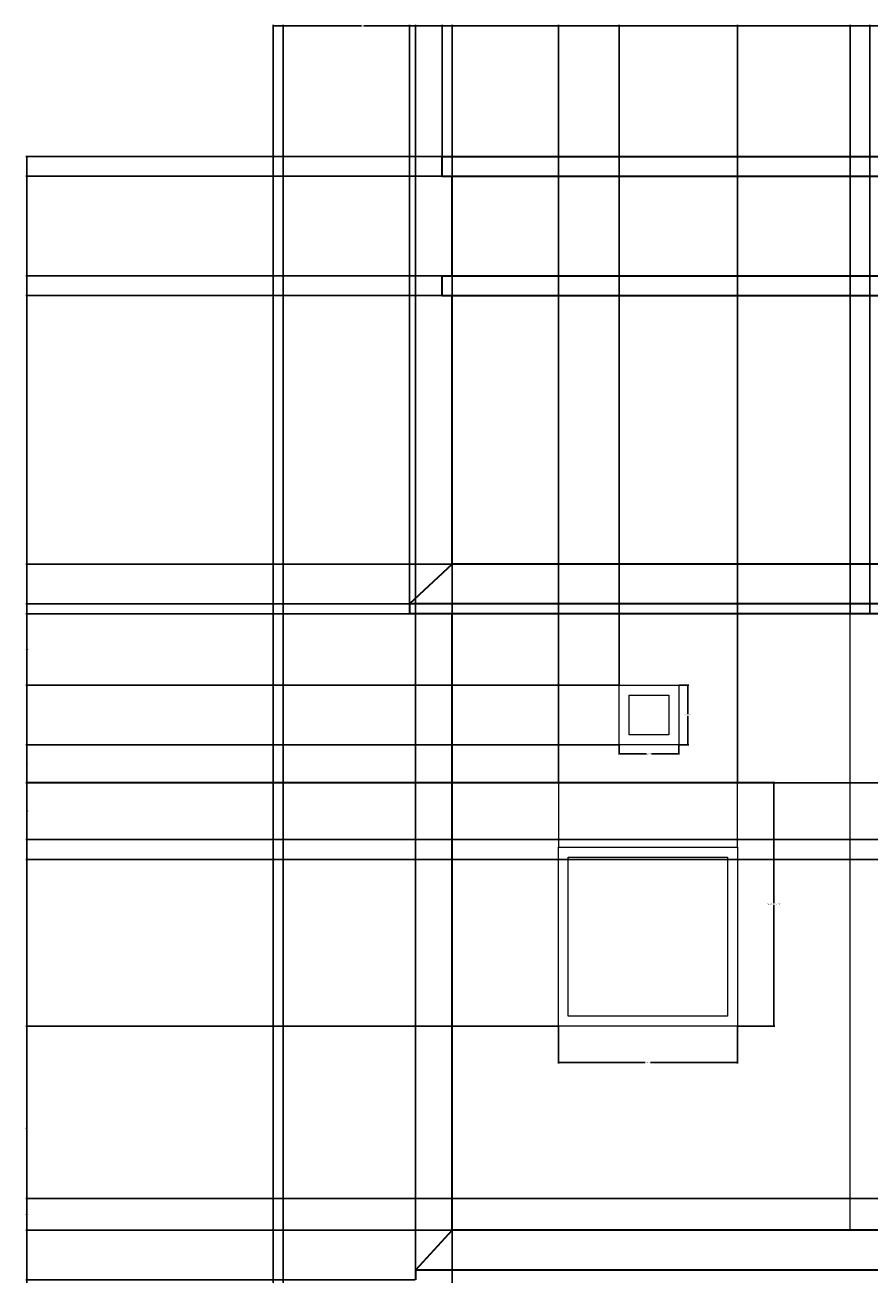
# Model space of a CAD drawing. Units: inches. Extents: x 1817 to 2378, y 1915 to 2370.
# Tile 4 of 8: x 1817 to 1987, y 2119 to 2370. Entities that reach past the tile are written whole.
import ezdxf

# ---------------------------------------------------------------- set-up
doc = ezdxf.new("R2010")
doc.units = ezdxf.units.IN
for name, color, linetype, lineweight in [('A-ANNO-DIMS', 2, 'Continuous', 18), ('A-ELEV', 7, 'Continuous', 35), ('A-GLAZ', 4, 'Continuous', 18), ('P-PIPE', 6, 'Continuous', 18)]:
    doc.layers.add(name, color=color, linetype=linetype, lineweight=lineweight)
doc.styles.get("Standard").update_dxf_attribs({"font": 'arial.ttf'})
doc.dimstyles.get("Standard").update_dxf_attribs({"dimtxt": 0.18, "dimasz": 0.18, "dimexe": 0.18, "dimexo": 0.0625, "dimgap": 0.09, "dimtad": 0, "dimtih": 1, "dimtoh": 1, "dimdec": 4, "dimzin": 0, "dimdsep": 46, "dimtxsty": 'Standard', "dimcen": 0.09, "dimadec": 0, "dimazin": 0, "dimtfac": 1, "dimtdec": 4, "dimtofl": 0, "dimtmove": 0, "dimatfit": 3, "dimfxl": 1, "dimtolj": 1, "dimtzin": 0, "dimarcsym": 0})

# ---------------------------------------------------------------- blocks, each defined once
blk = doc.blocks.new('WIN-SQ-900')
for points in [[(1924.43, 2204.58), (1960.43, 2204.58), (1960.43, 2217.58), (1924.43, 2217.58)], [(1924.43, 2204.58), (1960.43, 2204.58), (1960.43, 2168.58), (1924.43, 2168.58)], [(1926.43, 2202.58), (1958.43, 2202.58), (1958.43, 2170.58), (1926.43, 2170.58)]]:
    blk.add_lwpolyline(points, close=True)
blk = doc.blocks.new('VENT-300')
for points in [[(1936.66, 2237.16), (1948.66, 2237.16), (1948.66, 2225.16), (1936.66, 2225.16)], [(1938.66, 2235.16), (1946.66, 2235.16), (1946.66, 2227.16), (1938.66, 2227.16)]]:
    blk.add_lwpolyline(points, close=True)
blk = doc.blocks.new('*D4')
at = {"layer": 'A-ANNO-DIMS', "color": 0, "lineweight": -2, "transparency": 16777216}
for p, q in [((1960.49, 2217.58), (1967.96, 2217.58)), ((1967.78, 2217.4), (1967.78, 2193.27)), ((1967.78, 2168.76), (1967.78, 2192.89)), ((1960.49, 2168.58), (1967.96, 2168.58))]:
    blk.add_line(p, q, dxfattribs=at)
at = {"layer": 'A-ANNO-DIMS', "color": 0, "transparency": 16777216}
for points in [[(1967.75, 2217.4), (1967.81, 2217.4), (1967.78, 2217.58)], [(1967.75, 2168.76), (1967.81, 2168.76), (1967.78, 2168.58)]]:
    blk.add_solid(points, dxfattribs=at)
at = {"layer": 'Defpoints', "color": 0, "transparency": 16777216}
for p in [(1960.43, 2217.58), (1967.78, 2217.58), (1960.43, 2168.58)]:
    blk.add_point(p, dxfattribs=at)
at = {"layer": 'A-ANNO-DIMS', "color": 0, "transparency": 16777216, "insert": (1967.78, 2193.08), "char_height": 0.18, "attachment_point": 5}
blk.add_mtext('\\A1;SQUARE WINDOW 49 TYP.', dxfattribs=at)
blk = doc.blocks.new('*D5')
at = {"layer": 'A-ANNO-DIMS', "color": 0, "lineweight": -2, "transparency": 16777216}
for p, q in [((1924.43, 2168.52), (1924.43, 2161.05)), ((1960.43, 2168.52), (1960.43, 2161.05)), ((1924.61, 2161.23), (1941.9, 2161.23)), ((1960.25, 2161.23), (1942.95, 2161.23))]:
    blk.add_line(p, q, dxfattribs=at)
at = {"layer": 'A-ANNO-DIMS', "color": 0, "transparency": 16777216}
for points in [[(1924.61, 2161.26), (1924.61, 2161.2), (1924.43, 2161.23)], [(1960.25, 2161.26), (1960.25, 2161.2), (1960.43, 2161.23)]]:
    blk.add_solid(points, dxfattribs=at)
at = {"layer": 'Defpoints', "color": 0, "transparency": 16777216}
for p in [(1924.43, 2168.58), (1960.43, 2168.58), (1960.43, 2161.23)]:
    blk.add_point(p, dxfattribs=at)
at = {"layer": 'A-ANNO-DIMS', "color": 0, "transparency": 16777216, "insert": (1942.43, 2161.23), "char_height": 0.18, "attachment_point": 5}
blk.add_mtext('\\A1;36 TYP.', dxfattribs=at)
blk = doc.blocks.new('*D6')
at = {"layer": 'A-ANNO-DIMS', "color": 0, "lineweight": -2, "transparency": 16777216}
for p, q in [((1948.73, 2237.16), (1950.64, 2237.16)), ((1950.46, 2236.98), (1950.46, 2231.34)), ((1950.46, 2225.34), (1950.46, 2230.98)), ((1948.73, 2225.16), (1950.64, 2225.16))]:
    blk.add_line(p, q, dxfattribs=at)
at = {"layer": 'A-ANNO-DIMS', "color": 0, "transparency": 16777216}
for points in [[(1950.43, 2236.98), (1950.49, 2236.98), (1950.46, 2237.16)], [(1950.43, 2225.34), (1950.49, 2225.34), (1950.46, 2225.16)]]:
    blk.add_solid(points, dxfattribs=at)
at = {"layer": 'Defpoints', "color": 0, "transparency": 16777216}
for p in [(1948.66, 2237.16), (1950.46, 2237.16), (1948.66, 2225.16)]:
    blk.add_point(p, dxfattribs=at)
at = {"layer": 'A-ANNO-DIMS', "color": 0, "transparency": 16777216, "insert": (1950.46, 2231.16), "char_height": 0.18, "attachment_point": 5}
blk.add_mtext('\\A1;VENT 12 TYP.', dxfattribs=at)
blk = doc.blocks.new('*D7')
at = {"layer": 'A-ANNO-DIMS', "color": 0, "lineweight": -2, "transparency": 16777216}
for p, q in [((1936.66, 2225.1), (1936.66, 2223.18)), ((1936.84, 2223.36), (1942.15, 2223.36)), ((1948.48, 2223.36), (1943.18, 2223.36)), ((1948.66, 2225.1), (1948.66, 2223.18))]:
    blk.add_line(p, q, dxfattribs=at)
at = {"layer": 'A-ANNO-DIMS', "color": 0, "transparency": 16777216}
for points in [[(1936.84, 2223.39), (1936.84, 2223.33), (1936.66, 2223.36)], [(1948.48, 2223.39), (1948.48, 2223.33), (1948.66, 2223.36)]]:
    blk.add_solid(points, dxfattribs=at)
at = {"layer": 'Defpoints', "color": 0, "transparency": 16777216}
for p in [(1936.66, 2225.16), (1948.66, 2225.16), (1948.66, 2223.36)]:
    blk.add_point(p, dxfattribs=at)
at = {"layer": 'A-ANNO-DIMS', "color": 0, "transparency": 16777216, "insert": (1942.66, 2223.36), "char_height": 0.18, "attachment_point": 5}
blk.add_mtext('\\A1;12 TYP.', dxfattribs=at)
blk = doc.blocks.new('*D10')
at = {"layer": 'A-ANNO-DIMS', "color": 0, "lineweight": -2, "transparency": 16777216}
for p, q in [((1867.08, 2019.57), (1867.08, 2369.94)), ((1867.26, 2369.76), (1884.87, 2369.76)), ((1902.9, 2369.76), (1885.3, 2369.76)), ((1903.08, 2019.57), (1903.08, 2369.94))]:
    blk.add_line(p, q, dxfattribs=at)
at = {"layer": 'A-ANNO-DIMS', "color": 0, "transparency": 16777216}
for points in [[(1867.26, 2369.79), (1867.26, 2369.73), (1867.08, 2369.76)], [(1902.9, 2369.79), (1902.9, 2369.73), (1903.08, 2369.76)]]:
    blk.add_solid(points, dxfattribs=at)
at = {"layer": 'Defpoints', "color": 0, "transparency": 16777216}
for p in [(1903.08, 2369.76), (1867.08, 2019.51), (1903.08, 2019.51)]:
    blk.add_point(p, dxfattribs=at)
at = {"layer": 'A-ANNO-DIMS', "color": 0, "transparency": 16777216, "insert": (1885.08, 2369.76), "char_height": 0.18, "attachment_point": 5}
blk.add_mtext('\\A1;36', dxfattribs=at)
blk = doc.blocks.new('*D11')
at = {"layer": 'A-ANNO-DIMS', "color": 0, "lineweight": -2, "transparency": 16777216}
for p, q in [((1895.7, 2119.57), (1895.7, 2369.94)), ((1895.88, 2369.76), (1899, 2369.76)), ((1902.9, 2369.76), (1899.78, 2369.76)), ((1903.08, 2127.57), (1903.08, 2369.94))]:
    blk.add_line(p, q, dxfattribs=at)
at = {"layer": 'A-ANNO-DIMS', "color": 0, "transparency": 16777216}
for points in [[(1895.88, 2369.79), (1895.88, 2369.73), (1895.7, 2369.76)], [(1902.9, 2369.79), (1902.9, 2369.73), (1903.08, 2369.76)]]:
    blk.add_solid(points, dxfattribs=at)
at = {"layer": 'Defpoints', "color": 0, "transparency": 16777216}
for p in [(1903.08, 2369.76), (1903.08, 2127.51), (1895.7, 2119.51)]:
    blk.add_point(p, dxfattribs=at)
at = {"layer": 'A-ANNO-DIMS', "color": 0, "transparency": 16777216, "insert": (1899.39, 2369.76), "char_height": 0.18, "attachment_point": 5}
blk.add_mtext('\\A1;7.389', dxfattribs=at)
blk = doc.blocks.new('*D23')
at = {"layer": 'A-ANNO-DIMS', "color": 0, "lineweight": -2, "transparency": 16777216}
for p, q in [((2320.11, 2156.45), (2320.11, 1915.08)), ((1867.08, 1965.45), (1867.08, 1915.08)), ((1867.26, 1915.26), (2093.3, 1915.26)), ((2319.93, 1915.26), (2093.89, 1915.26))]:
    blk.add_line(p, q, dxfattribs=at)
at = {"layer": 'A-ANNO-DIMS', "color": 0, "transparency": 16777216}
for points in [[(1867.26, 1915.29), (1867.26, 1915.23), (1867.08, 1915.26)], [(2319.93, 1915.29), (2319.93, 1915.23), (2320.11, 1915.26)]]:
    blk.add_solid(points, dxfattribs=at)
at = {"layer": 'Defpoints', "color": 0, "transparency": 16777216}
for p in [(2320.11, 2156.51), (1867.08, 1965.51), (2320.11, 1915.26)]:
    blk.add_point(p, dxfattribs=at)
at = {"layer": 'A-ANNO-DIMS', "color": 0, "transparency": 16777216, "insert": (2093.6, 1915.26), "char_height": 0.18, "attachment_point": 5}
blk.add_mtext('\\A1;453', dxfattribs=at)
blk = doc.blocks.new('*D25')
at = {"layer": 'A-ANNO-DIMS', "color": 0, "lineweight": -2, "transparency": 16777216}
for p, q in [((1903.08, 2127.57), (1903.08, 2369.94)), ((1903.26, 2369.76), (1913.36, 2369.76)), ((1924.25, 2369.76), (1914.15, 2369.76)), ((1924.43, 2217.64), (1924.43, 2369.94))]:
    blk.add_line(p, q, dxfattribs=at)
at = {"layer": 'A-ANNO-DIMS', "color": 0, "transparency": 16777216}
for points in [[(1903.26, 2369.79), (1903.26, 2369.73), (1903.08, 2369.76)], [(1924.25, 2369.79), (1924.25, 2369.73), (1924.43, 2369.76)]]:
    blk.add_solid(points, dxfattribs=at)
at = {"layer": 'Defpoints', "color": 0, "transparency": 16777216}
for p in [(1924.43, 2369.76), (1924.43, 2217.58), (1903.08, 2127.51)]:
    blk.add_point(p, dxfattribs=at)
at = {"layer": 'A-ANNO-DIMS', "color": 0, "transparency": 16777216, "insert": (1913.76, 2369.76), "char_height": 0.18, "attachment_point": 5}
blk.add_mtext('\\A1;21.34', dxfattribs=at)
blk = doc.blocks.new('*D26')
at = {"layer": 'A-ANNO-DIMS', "color": 0, "lineweight": -2, "transparency": 16777216}
for p, q in [((1924.43, 2217.64), (1924.43, 2369.94)), ((1924.61, 2369.76), (1930.16, 2369.76)), ((1936.48, 2369.76), (1930.93, 2369.76)), ((1936.66, 2237.22), (1936.66, 2369.94))]:
    blk.add_line(p, q, dxfattribs=at)
at = {"layer": 'A-ANNO-DIMS', "color": 0, "transparency": 16777216}
for points in [[(1924.61, 2369.79), (1924.61, 2369.73), (1924.43, 2369.76)], [(1936.48, 2369.79), (1936.48, 2369.73), (1936.66, 2369.76)]]:
    blk.add_solid(points, dxfattribs=at)
at = {"layer": 'Defpoints', "color": 0, "transparency": 16777216}
for p in [(1936.66, 2369.76), (1936.66, 2237.16), (1924.43, 2217.58)]:
    blk.add_point(p, dxfattribs=at)
at = {"layer": 'A-ANNO-DIMS', "color": 0, "transparency": 16777216, "insert": (1930.55, 2369.76), "char_height": 0.18, "attachment_point": 5}
blk.add_mtext('\\A1;12.24', dxfattribs=at)
blk = doc.blocks.new('*D27')
at = {"layer": 'A-ANNO-DIMS', "color": 0, "lineweight": -2, "transparency": 16777216}
for p, q in [((1936.66, 2237.22), (1936.66, 2369.94)), ((1936.84, 2369.76), (1948.15, 2369.76)), ((1960.25, 2369.76), (1948.94, 2369.76)), ((1960.43, 2217.64), (1960.43, 2369.94))]:
    blk.add_line(p, q, dxfattribs=at)
at = {"layer": 'A-ANNO-DIMS', "color": 0, "transparency": 16777216}
for points in [[(1936.84, 2369.79), (1936.84, 2369.73), (1936.66, 2369.76)], [(1960.25, 2369.79), (1960.25, 2369.73), (1960.43, 2369.76)]]:
    blk.add_solid(points, dxfattribs=at)
at = {"layer": 'Defpoints', "color": 0, "transparency": 16777216}
for p in [(1960.43, 2369.76), (1936.66, 2237.16), (1960.43, 2217.58)]:
    blk.add_point(p, dxfattribs=at)
at = {"layer": 'A-ANNO-DIMS', "color": 0, "transparency": 16777216, "insert": (1948.55, 2369.76), "char_height": 0.18, "attachment_point": 5}
blk.add_mtext('\\A1;23.76', dxfattribs=at)
blk = doc.blocks.new('*D28')
at = {"layer": 'A-ANNO-DIMS', "color": 0, "lineweight": -2, "transparency": 16777216}
for p, q in [((1960.43, 2217.64), (1960.43, 2369.94)), ((1960.61, 2369.76), (1971.36, 2369.76)), ((1982.9, 2369.76), (1972.15, 2369.76)), ((1983.08, 2251.57), (1983.08, 2369.94))]:
    blk.add_line(p, q, dxfattribs=at)
at = {"layer": 'A-ANNO-DIMS', "color": 0, "transparency": 16777216}
for points in [[(1960.61, 2369.79), (1960.61, 2369.73), (1960.43, 2369.76)], [(1982.9, 2369.79), (1982.9, 2369.73), (1983.08, 2369.76)]]:
    blk.add_solid(points, dxfattribs=at)
at = {"layer": 'Defpoints', "color": 0, "transparency": 16777216}
for p in [(1983.08, 2369.76), (1983.08, 2251.51), (1960.43, 2217.58)]:
    blk.add_point(p, dxfattribs=at)
at = {"layer": 'A-ANNO-DIMS', "color": 0, "transparency": 16777216, "insert": (1971.76, 2369.76), "char_height": 0.18, "attachment_point": 5}
blk.add_mtext('\\A1;22.66', dxfattribs=at)
blk = doc.blocks.new('*D29')
at = {"layer": 'A-ANNO-DIMS', "color": 0, "lineweight": -2, "transparency": 16777216}
for p, q in [((1983.08, 2251.57), (1983.08, 2369.94)), ((1983.26, 2369.76), (1984.93, 2369.76)), ((1986.9, 2369.76), (1985.24, 2369.76)), ((1987.08, 2251.57), (1987.08, 2369.94))]:
    blk.add_line(p, q, dxfattribs=at)
at = {"layer": 'A-ANNO-DIMS', "color": 0, "transparency": 16777216}
for points in [[(1983.26, 2369.79), (1983.26, 2369.73), (1983.08, 2369.76)], [(1986.9, 2369.79), (1986.9, 2369.73), (1987.08, 2369.76)]]:
    blk.add_solid(points, dxfattribs=at)
at = {"layer": 'Defpoints', "color": 0, "transparency": 16777216}
for p in [(1987.08, 2369.76), (1983.08, 2251.51), (1987.08, 2251.51)]:
    blk.add_point(p, dxfattribs=at)
at = {"layer": 'A-ANNO-DIMS', "color": 0, "transparency": 16777216, "insert": (1985.08, 2369.76), "char_height": 0.18, "attachment_point": 5}
blk.add_mtext('\\A1;4', dxfattribs=at)
blk = doc.blocks.new('*D30')
at = {"layer": 'A-ANNO-DIMS', "color": 0, "lineweight": -2, "transparency": 16777216}
for p, q in [((1987.08, 2251.57), (1987.08, 2369.94)), ((1987.26, 2369.76), (1996.86, 2369.76)), ((2006.9, 2369.76), (1997.31, 2369.76)), ((2007.08, 2251.57), (2007.08, 2369.94))]:
    blk.add_line(p, q, dxfattribs=at)
at = {"layer": 'A-ANNO-DIMS', "color": 0, "transparency": 16777216}
for points in [[(1987.26, 2369.79), (1987.26, 2369.73), (1987.08, 2369.76)], [(2006.9, 2369.79), (2006.9, 2369.73), (2007.08, 2369.76)]]:
    blk.add_solid(points, dxfattribs=at)
at = {"layer": 'Defpoints', "color": 0, "transparency": 16777216}
for p in [(2007.08, 2369.76), (1987.08, 2251.51), (2007.08, 2251.51)]:
    blk.add_point(p, dxfattribs=at)
at = {"layer": 'A-ANNO-DIMS', "color": 0, "transparency": 16777216, "insert": (1997.08, 2369.76), "char_height": 0.18, "attachment_point": 5}
blk.add_mtext('\\A1;20', dxfattribs=at)
blk = doc.blocks.new('*D42')
at = {"layer": 'A-ANNO-DIMS', "color": 0, "lineweight": -2, "transparency": 16777216}
for p, q in [((1894.51, 2253.57), (1894.51, 2369.94)), ((1894.69, 2369.76), (1898.4, 2369.76)), ((1902.9, 2369.76), (1899.19, 2369.76)), ((1903.08, 2261.57), (1903.08, 2369.94))]:
    blk.add_line(p, q, dxfattribs=at)
at = {"layer": 'A-ANNO-DIMS', "color": 0, "transparency": 16777216}
for points in [[(1894.69, 2369.79), (1894.69, 2369.73), (1894.51, 2369.76)], [(1902.9, 2369.79), (1902.9, 2369.73), (1903.08, 2369.76)]]:
    blk.add_solid(points, dxfattribs=at)
at = {"layer": 'Defpoints', "color": 0, "transparency": 16777216}
for p in [(1903.08, 2369.76), (1903.08, 2261.51), (1894.51, 2253.51)]:
    blk.add_point(p, dxfattribs=at)
at = {"layer": 'A-ANNO-DIMS', "color": 0, "transparency": 16777216, "insert": (1898.8, 2369.76), "char_height": 0.18, "attachment_point": 5}
blk.add_mtext('\\A1;8.579', dxfattribs=at)
blk = doc.blocks.new('*D43')
at = {"layer": 'A-ANNO-DIMS', "color": 0, "lineweight": -2, "transparency": 16777216}
for p, q in [((1901.08, 2343.57), (1901.08, 2369.94)), ((1901.26, 2369.76), (1901.94, 2369.76)), ((1902.9, 2369.76), (1902.23, 2369.76)), ((1903.08, 2339.57), (1903.08, 2369.94))]:
    blk.add_line(p, q, dxfattribs=at)
at = {"layer": 'A-ANNO-DIMS', "color": 0, "transparency": 16777216}
for points in [[(1901.26, 2369.79), (1901.26, 2369.73), (1901.08, 2369.76)], [(1902.9, 2369.79), (1902.9, 2369.73), (1903.08, 2369.76)]]:
    blk.add_solid(points, dxfattribs=at)
at = {"layer": 'Defpoints', "color": 0, "transparency": 16777216}
for p in [(1903.08, 2369.76), (1901.08, 2343.51), (1903.08, 2339.51)]:
    blk.add_point(p, dxfattribs=at)
at = {"layer": 'A-ANNO-DIMS', "color": 0, "transparency": 16777216, "insert": (1902.08, 2369.76), "char_height": 0.18, "attachment_point": 5}
blk.add_mtext('\\A1;2', dxfattribs=at)
blk = doc.blocks.new('*D44')
at = {"layer": 'A-ANNO-DIMS', "color": 0, "lineweight": -2, "transparency": 16777216}
for p, q in [((1903.08, 2261.57), (1903.08, 2369.94)), ((1903.26, 2369.76), (1954.8, 2369.76)), ((2006.9, 2369.76), (1955.36, 2369.76)), ((2007.08, 2291.57), (2007.08, 2369.94))]:
    blk.add_line(p, q, dxfattribs=at)
at = {"layer": 'A-ANNO-DIMS', "color": 0, "transparency": 16777216}
for points in [[(1903.26, 2369.79), (1903.26, 2369.73), (1903.08, 2369.76)], [(2006.9, 2369.79), (2006.9, 2369.73), (2007.08, 2369.76)]]:
    blk.add_solid(points, dxfattribs=at)
at = {"layer": 'Defpoints', "color": 0, "transparency": 16777216}
for p in [(2007.08, 2369.76), (2007.08, 2291.51), (1903.08, 2261.51)]:
    blk.add_point(p, dxfattribs=at)
at = {"layer": 'A-ANNO-DIMS', "color": 0, "transparency": 16777216, "insert": (1955.08, 2369.76), "char_height": 0.18, "attachment_point": 5}
blk.add_mtext('\\A1;104', dxfattribs=at)
blk = doc.blocks.new('*D51')
at = {"layer": 'A-ANNO-DIMS', "color": 0, "lineweight": -2, "transparency": 16777216}
for p, q in [((2281.02, 2261.51), (1817.4, 2261.51)), ((1817.58, 2261.33), (1817.58, 2257.69)), ((1817.58, 2253.69), (1817.58, 2257.33)), ((2289.54, 2253.51), (1817.4, 2253.51))]:
    blk.add_line(p, q, dxfattribs=at)
at = {"layer": 'A-ANNO-DIMS', "color": 0, "transparency": 16777216}
for points in [[(1817.55, 2261.33), (1817.61, 2261.33), (1817.58, 2261.51)], [(1817.55, 2253.69), (1817.61, 2253.69), (1817.58, 2253.51)]]:
    blk.add_solid(points, dxfattribs=at)
at = {"layer": 'Defpoints', "color": 0, "transparency": 16777216}
for p in [(1817.58, 2261.51), (2281.08, 2261.51), (2289.61, 2253.51)]:
    blk.add_point(p, dxfattribs=at)
at = {"layer": 'A-ANNO-DIMS', "color": 0, "transparency": 16777216, "insert": (1817.58, 2257.51), "char_height": 0.18, "attachment_point": 5}
blk.add_mtext('\\A1;8', dxfattribs=at)
blk = doc.blocks.new('*D54')
at = {"layer": 'A-ANNO-DIMS', "color": 0, "lineweight": -2, "transparency": 16777216}
for p, q in [((1901.02, 2343.51), (1817.4, 2343.51)), ((1817.58, 2343.33), (1817.58, 2154.69)), ((1817.58, 1965.69), (1817.58, 2154.33)), ((1867.02, 1965.51), (1817.4, 1965.51))]:
    blk.add_line(p, q, dxfattribs=at)
at = {"layer": 'A-ANNO-DIMS', "color": 0, "transparency": 16777216}
for points in [[(1817.55, 2343.33), (1817.61, 2343.33), (1817.58, 2343.51)], [(1817.55, 1965.69), (1817.61, 1965.69), (1817.58, 1965.51)]]:
    blk.add_solid(points, dxfattribs=at)
at = {"layer": 'Defpoints', "color": 0, "transparency": 16777216}
for p in [(1817.58, 2343.51), (1901.08, 2343.51), (1867.08, 1965.51)]:
    blk.add_point(p, dxfattribs=at)
at = {"layer": 'A-ANNO-DIMS', "color": 0, "transparency": 16777216, "insert": (1817.58, 2154.51), "char_height": 0.18, "attachment_point": 5}
blk.add_mtext('\\A1;378', dxfattribs=at)
blk = doc.blocks.new('*D60')
at = {"layer": 'A-ANNO-DIMS', "color": 0, "lineweight": -2, "transparency": 16777216}
for p, q in [((1903.02, 2127.51), (1817.4, 2127.51)), ((1817.58, 2127.33), (1817.58, 2122.69)), ((1817.58, 2117.69), (1817.58, 2122.33)), ((1895.63, 2117.51), (1817.4, 2117.51))]:
    blk.add_line(p, q, dxfattribs=at)
at = {"layer": 'A-ANNO-DIMS', "color": 0, "transparency": 16777216}
for points in [[(1817.55, 2127.33), (1817.61, 2127.33), (1817.58, 2127.51)], [(1817.55, 2117.69), (1817.61, 2117.69), (1817.58, 2117.51)]]:
    blk.add_solid(points, dxfattribs=at)
at = {"layer": 'Defpoints', "color": 0, "transparency": 16777216}
for p in [(1817.58, 2127.51), (1903.08, 2127.51), (1895.7, 2117.51)]:
    blk.add_point(p, dxfattribs=at)
at = {"layer": 'A-ANNO-DIMS', "color": 0, "transparency": 16777216, "insert": (1817.58, 2122.51), "char_height": 0.18, "attachment_point": 5}
blk.add_mtext('\\A1;10', dxfattribs=at)
blk = doc.blocks.new('*D61')
at = {"layer": 'A-ANNO-DIMS', "color": 0, "lineweight": -2, "transparency": 16777216}
for p, q in [((1924.36, 2168.58), (1817.4, 2168.58)), ((1817.58, 2168.4), (1817.58, 2148.23)), ((1817.58, 2127.69), (1817.58, 2147.86)), ((1903.02, 2127.51), (1817.4, 2127.51))]:
    blk.add_line(p, q, dxfattribs=at)
at = {"layer": 'A-ANNO-DIMS', "color": 0, "transparency": 16777216}
for points in [[(1817.55, 2168.4), (1817.61, 2168.4), (1817.58, 2168.58)], [(1817.55, 2127.69), (1817.61, 2127.69), (1817.58, 2127.51)]]:
    blk.add_solid(points, dxfattribs=at)
at = {"layer": 'Defpoints', "color": 0, "transparency": 16777216}
for p in [(1817.58, 2168.58), (1924.43, 2168.58), (1903.08, 2127.51)]:
    blk.add_point(p, dxfattribs=at)
at = {"layer": 'A-ANNO-DIMS', "color": 0, "transparency": 16777216, "insert": (1817.58, 2148.05), "char_height": 0.18, "attachment_point": 5}
blk.add_mtext('\\A1;41.07', dxfattribs=at)
blk = doc.blocks.new('*D62')
at = {"layer": 'A-ANNO-DIMS', "color": 0, "lineweight": -2, "transparency": 16777216}
for p, q in [((1936.6, 2225.16), (1817.4, 2225.16)), ((1817.58, 2224.98), (1817.58, 2221.55)), ((1817.58, 2217.76), (1817.58, 2221.19)), ((1924.36, 2217.58), (1817.4, 2217.58))]:
    blk.add_line(p, q, dxfattribs=at)
at = {"layer": 'A-ANNO-DIMS', "color": 0, "transparency": 16777216}
for points in [[(1817.55, 2224.98), (1817.61, 2224.98), (1817.58, 2225.16)], [(1817.55, 2217.76), (1817.61, 2217.76), (1817.58, 2217.58)]]:
    blk.add_solid(points, dxfattribs=at)
at = {"layer": 'Defpoints', "color": 0, "transparency": 16777216}
for p in [(1817.58, 2225.16), (1936.66, 2225.16), (1924.43, 2217.58)]:
    blk.add_point(p, dxfattribs=at)
at = {"layer": 'A-ANNO-DIMS', "color": 0, "transparency": 16777216, "insert": (1817.58, 2221.37), "char_height": 0.18, "attachment_point": 5}
blk.add_mtext('\\A1;7.578', dxfattribs=at)
blk = doc.blocks.new('*D63')
at = {"layer": 'A-ANNO-DIMS', "color": 0, "lineweight": -2, "transparency": 16777216}
for p, q in [((1903.02, 2251.51), (1817.4, 2251.51)), ((1817.58, 2251.33), (1817.58, 2244.52)), ((1817.58, 2237.34), (1817.58, 2244.15)), ((1936.6, 2237.16), (1817.4, 2237.16))]:
    blk.add_line(p, q, dxfattribs=at)
at = {"layer": 'A-ANNO-DIMS', "color": 0, "transparency": 16777216}
for points in [[(1817.55, 2251.33), (1817.61, 2251.33), (1817.58, 2251.51)], [(1817.55, 2237.34), (1817.61, 2237.34), (1817.58, 2237.16)]]:
    blk.add_solid(points, dxfattribs=at)
at = {"layer": 'Defpoints', "color": 0, "transparency": 16777216}
for p in [(1817.58, 2251.51), (1903.08, 2251.51), (1936.66, 2237.16)]:
    blk.add_point(p, dxfattribs=at)
at = {"layer": 'A-ANNO-DIMS', "color": 0, "transparency": 16777216, "insert": (1817.58, 2244.33), "char_height": 0.18, "attachment_point": 5}
blk.add_mtext('\\A1;14.35', dxfattribs=at)
blk = doc.blocks.new('*D64')
at = {"layer": 'A-ANNO-DIMS', "color": 0, "lineweight": -2, "transparency": 16777216}
for p, q in [((1903.02, 2261.51), (1817.4, 2261.51)), ((1817.58, 2261.33), (1817.58, 2256.69)), ((1817.58, 2251.69), (1817.58, 2256.33)), ((1894.44, 2251.51), (1817.4, 2251.51))]:
    blk.add_line(p, q, dxfattribs=at)
at = {"layer": 'A-ANNO-DIMS', "color": 0, "transparency": 16777216}
for points in [[(1817.55, 2261.33), (1817.61, 2261.33), (1817.58, 2261.51)], [(1817.55, 2251.69), (1817.61, 2251.69), (1817.58, 2251.51)]]:
    blk.add_solid(points, dxfattribs=at)
at = {"layer": 'Defpoints', "color": 0, "transparency": 16777216}
for p in [(1817.58, 2261.51), (1903.08, 2261.51), (1894.51, 2251.51)]:
    blk.add_point(p, dxfattribs=at)
at = {"layer": 'A-ANNO-DIMS', "color": 0, "transparency": 16777216, "insert": (1817.58, 2256.51), "char_height": 0.18, "attachment_point": 5}
blk.add_mtext('\\A1;10', dxfattribs=at)
blk = doc.blocks.new('*D65')
at = {"layer": 'A-ANNO-DIMS', "color": 0, "lineweight": -2, "transparency": 16777216}
for p, q in [((1901.02, 2315.51), (1817.4, 2315.51)), ((1817.58, 2315.33), (1817.58, 2288.69)), ((1817.58, 2261.69), (1817.58, 2288.33)), ((1903.02, 2261.51), (1817.4, 2261.51))]:
    blk.add_line(p, q, dxfattribs=at)
at = {"layer": 'A-ANNO-DIMS', "color": 0, "transparency": 16777216}
for points in [[(1817.55, 2315.33), (1817.61, 2315.33), (1817.58, 2315.51)], [(1817.55, 2261.69), (1817.61, 2261.69), (1817.58, 2261.51)]]:
    blk.add_solid(points, dxfattribs=at)
at = {"layer": 'Defpoints', "color": 0, "transparency": 16777216}
for p in [(1817.58, 2315.51), (1901.08, 2315.51), (1903.08, 2261.51)]:
    blk.add_point(p, dxfattribs=at)
at = {"layer": 'A-ANNO-DIMS', "color": 0, "transparency": 16777216, "insert": (1817.58, 2288.51), "char_height": 0.18, "attachment_point": 5}
blk.add_mtext('\\A1;54', dxfattribs=at)
blk = doc.blocks.new('*D66')
at = {"layer": 'A-ANNO-DIMS', "color": 0, "lineweight": -2, "transparency": 16777216}
for p, q in [((1901.022352, 2319.508728), (1817.404024, 2319.508728)), ((1817.584024, 2319.328728), (1817.584024, 2317.688728)), ((1817.584024, 2315.688728), (1817.584024, 2317.328728)), ((1901.022352, 2315.508728), (1817.404024, 2315.508728))]:
    blk.add_line(p, q, dxfattribs=at)
at = {"layer": 'A-ANNO-DIMS', "color": 0, "transparency": 16777216}
for points in [[(1817.554024, 2319.328728), (1817.614024, 2319.328728), (1817.584024, 2319.508728)], [(1817.554024, 2315.688728), (1817.614024, 2315.688728), (1817.584024, 2315.508728)]]:
    blk.add_solid(points, dxfattribs=at)
at = {"layer": 'Defpoints', "color": 0, "transparency": 16777216}
for p in [(1817.584024, 2319.508728), (1901.084852, 2319.508728), (1901.084852, 2315.508728)]:
    blk.add_point(p, dxfattribs=at)
at = {"layer": 'A-ANNO-DIMS', "color": 0, "transparency": 16777216, "insert": (1817.584024, 2317.508728), "char_height": 0.18, "attachment_point": 5}
blk.add_mtext('\\A1;4', dxfattribs=at)
blk = doc.blocks.new('*D67')
at = {"layer": 'A-ANNO-DIMS', "color": 0, "lineweight": -2, "transparency": 16777216}
for p, q in [((1901.02, 2339.51), (1817.4, 2339.51)), ((1817.58, 2339.33), (1817.58, 2329.69)), ((1817.58, 2319.69), (1817.58, 2329.33)), ((1901.02, 2319.51), (1817.4, 2319.51))]:
    blk.add_line(p, q, dxfattribs=at)
at = {"layer": 'A-ANNO-DIMS', "color": 0, "transparency": 16777216}
for points in [[(1817.55, 2339.33), (1817.61, 2339.33), (1817.58, 2339.51)], [(1817.55, 2319.69), (1817.61, 2319.69), (1817.58, 2319.51)]]:
    blk.add_solid(points, dxfattribs=at)
at = {"layer": 'Defpoints', "color": 0, "transparency": 16777216}
for p in [(1817.58, 2339.51), (1901.08, 2339.51), (1901.08, 2319.51)]:
    blk.add_point(p, dxfattribs=at)
at = {"layer": 'A-ANNO-DIMS', "color": 0, "transparency": 16777216, "insert": (1817.58, 2329.51), "char_height": 0.18, "attachment_point": 5}
blk.add_mtext('\\A1;20', dxfattribs=at)
blk = doc.blocks.new('*D68')
at = {"layer": 'A-ANNO-DIMS', "color": 0, "lineweight": -2, "transparency": 16777216}
for p, q in [((1901.022352, 2343.508728), (1817.404024, 2343.508728)), ((1817.584024, 2343.328728), (1817.584024, 2341.688728)), ((1817.584024, 2339.688728), (1817.584024, 2341.328728)), ((1901.022352, 2339.508728), (1817.404024, 2339.508728))]:
    blk.add_line(p, q, dxfattribs=at)
at = {"layer": 'A-ANNO-DIMS', "color": 0, "transparency": 16777216}
for points in [[(1817.554024, 2343.328728), (1817.614024, 2343.328728), (1817.584024, 2343.508728)], [(1817.554024, 2339.688728), (1817.614024, 2339.688728), (1817.584024, 2339.508728)]]:
    blk.add_solid(points, dxfattribs=at)
at = {"layer": 'Defpoints', "color": 0, "transparency": 16777216}
for p in [(1817.584024, 2343.508728), (1901.084852, 2343.508728), (1901.084852, 2339.508728)]:
    blk.add_point(p, dxfattribs=at)
at = {"layer": 'A-ANNO-DIMS', "color": 0, "transparency": 16777216, "insert": (1817.584024, 2341.508728), "char_height": 0.18, "attachment_point": 5}
blk.add_mtext('\\A1;4', dxfattribs=at)
blk = doc.blocks.new('*D82')
at = {"layer": 'A-ANNO-DIMS', "color": 0, "lineweight": -2, "transparency": 16777216}
for p, q in [((2123.56, 2133.9), (1817.4, 2133.9)), ((1817.58, 2133.72), (1817.58, 2130.88)), ((1817.58, 2127.69), (1817.58, 2130.52)), ((2198.53, 2127.51), (1817.4, 2127.51))]:
    blk.add_line(p, q, dxfattribs=at)
at = {"layer": 'A-ANNO-DIMS', "color": 0, "transparency": 16777216}
for points in [[(1817.55, 2133.72), (1817.61, 2133.72), (1817.58, 2133.9)], [(1817.55, 2127.69), (1817.61, 2127.69), (1817.58, 2127.51)]]:
    blk.add_solid(points, dxfattribs=at)
at = {"layer": 'Defpoints', "color": 0, "transparency": 16777216}
for p in [(1817.58, 2133.9), (2123.62, 2133.9), (2198.59, 2127.51)]:
    blk.add_point(p, dxfattribs=at)
at = {"layer": 'A-ANNO-DIMS', "color": 0, "transparency": 16777216, "insert": (1817.58, 2130.7), "char_height": 0.18, "attachment_point": 5}
blk.add_mtext('\\A1;6.387', dxfattribs=at)
blk = doc.blocks.new('*D104')
at = {"layer": 'A-ANNO-DIMS', "color": 0, "lineweight": -2, "transparency": 16777216}
for p, q in [((2210.55, 2217.51), (1817.4, 2217.51)), ((1817.58, 2217.33), (1817.58, 2211.97)), ((1817.58, 2206.26), (1817.58, 2211.61)), ((2210.55, 2206.08), (1817.4, 2206.08))]:
    blk.add_line(p, q, dxfattribs=at)
at = {"layer": 'A-ANNO-DIMS', "color": 0, "transparency": 16777216}
for points in [[(1817.55, 2217.33), (1817.61, 2217.33), (1817.58, 2217.51)], [(1817.55, 2206.26), (1817.61, 2206.26), (1817.58, 2206.08)]]:
    blk.add_solid(points, dxfattribs=at)
at = {"layer": 'Defpoints', "color": 0, "transparency": 16777216}
for p in [(2210.62, 2217.51), (1817.58, 2206.08), (2210.62, 2206.08)]:
    blk.add_point(p, dxfattribs=at)
at = {"layer": 'A-ANNO-DIMS', "color": 0, "transparency": 16777216, "insert": (1817.58, 2211.79), "char_height": 0.18, "attachment_point": 5}
blk.add_mtext('\\A1;11.433', dxfattribs=at)
blk = doc.blocks.new('*D105')
at = {"layer": 'A-ANNO-DIMS', "color": 0, "lineweight": -2, "transparency": 16777216}
for p, q in [((2210.55, 2206.08), (1817.4, 2206.08)), ((1817.58, 2205.9), (1817.58, 2204.26)), ((1817.58, 2202.26), (1817.58, 2203.89)), ((2214.55, 2202.08), (1817.4, 2202.08))]:
    blk.add_line(p, q, dxfattribs=at)
at = {"layer": 'A-ANNO-DIMS', "color": 0, "transparency": 16777216}
for points in [[(1817.55, 2205.9), (1817.61, 2205.9), (1817.58, 2206.08)], [(1817.55, 2202.26), (1817.61, 2202.26), (1817.58, 2202.08)]]:
    blk.add_solid(points, dxfattribs=at)
at = {"layer": 'Defpoints', "color": 0, "transparency": 16777216}
for p in [(2210.62, 2206.08), (1817.58, 2202.08), (2214.62, 2202.08)]:
    blk.add_point(p, dxfattribs=at)
at = {"layer": 'A-ANNO-DIMS', "color": 0, "transparency": 16777216, "insert": (1817.58, 2204.08), "char_height": 0.18, "attachment_point": 5}
blk.add_mtext('\\A1;4.00', dxfattribs=at)
blk = doc.blocks.new('*D116')
at = {"layer": 'A-ANNO-DIMS', "color": 0, "lineweight": -2, "transparency": 16777216}
for p, q in [((1867.08, 2017.57), (1867.08, 2369.94)), ((1867.26, 2369.76), (1867.76, 2369.76)), ((1868.9, 2369.76), (1868.41, 2369.76)), ((1869.08, 2017.57), (1869.08, 2369.94))]:
    blk.add_line(p, q, dxfattribs=at)
at = {"layer": 'A-ANNO-DIMS', "color": 0, "transparency": 16777216}
for points in [[(1867.26, 2369.79), (1867.26, 2369.73), (1867.08, 2369.76)], [(1868.9, 2369.79), (1868.9, 2369.73), (1869.08, 2369.76)]]:
    blk.add_solid(points, dxfattribs=at)
at = {"layer": 'Defpoints', "color": 0, "transparency": 16777216}
for p in [(1869.08, 2369.76), (1867.08, 2017.51), (1869.08, 2017.51)]:
    blk.add_point(p, dxfattribs=at)
at = {"layer": 'A-ANNO-DIMS', "color": 0, "transparency": 16777216, "insert": (1868.08, 2369.76), "char_height": 0.18, "attachment_point": 5}
blk.add_mtext('\\A1;2.00', dxfattribs=at)
blk = doc.blocks.new('*D119')
at = {"layer": 'A-ANNO-DIMS', "color": 0, "lineweight": -2, "transparency": 16777216}
for p, q in [((1903.08, 1989.57), (1903.08, 2369.94)), ((1903.26, 2369.76), (2091.62, 2369.76)), ((2280.9, 2369.76), (2092.55, 2369.76)), ((2281.08, 1989.57), (2281.08, 2369.94))]:
    blk.add_line(p, q, dxfattribs=at)
at = {"layer": 'A-ANNO-DIMS', "color": 0, "transparency": 16777216}
for points in [[(1903.26, 2369.79), (1903.26, 2369.73), (1903.08, 2369.76)], [(2280.9, 2369.79), (2280.9, 2369.73), (2281.08, 2369.76)]]:
    blk.add_solid(points, dxfattribs=at)
at = {"layer": 'Defpoints', "color": 0, "transparency": 16777216}
for p in [(2281.08, 2369.76), (1903.08, 1989.51), (2281.08, 1989.51)]:
    blk.add_point(p, dxfattribs=at)
at = {"layer": 'A-ANNO-DIMS', "color": 0, "transparency": 16777216, "insert": (2092.08, 2369.76), "char_height": 0.18, "attachment_point": 5}
blk.add_mtext('\\A1;378.00', dxfattribs=at)

msp = doc.modelspace()

# ---------------------------------------------------------------- linework, layer by layer
at = {"layer": 'A-ELEV'}
for p, q in [((1901.0849, 2343.5087), (2127.0849, 2343.5087)), ((1901.0849, 2339.5087), (1901.0849, 2343.5087)), ((1901.0849, 2339.5087), (2127.0849, 2339.5087)), ((1903.0849, 2319.5087), (1903.0849, 2339.5087)), ((1901.0849, 2319.5087), (2009.0849, 2319.5087)), ((1901.0849, 2315.5087), (1901.0849, 2319.5087)), ((1901.0849, 2315.5087), (2009.0849, 2315.5087)), ((1903.0849, 2261.5087), (1903.0849, 2315.5087)), ((1903.0849, 2261.5087), (1894.506, 2253.5087)), ((2281.0849, 2261.5087), (1903.0849, 2261.5087)), ((2289.6055, 2253.5087), (1894.506, 2253.5087)), ((1894.506, 2253.5087), (1894.506, 2251.5087)), ((2289.6055, 2251.5087), (1894.506, 2251.5087)), ((1903.0849, 2127.5087), (1903.0849, 2251.5087)), ((1903.0849, 2127.5087), (1895.6961, 2119.5087)), ((2198.5896, 2127.5087), (1903.0849, 2127.5087)), ((2198.5896, 2119.5087), (1895.6961, 2119.5087)), ((1895.6961, 2119.5087), (1895.6961, 2117.5087))]:
    msp.add_line(p, q, dxfattribs=at)
at = {"layer": 'P-PIPE'}
msp.add_line((1983.0849, 2127.5087), (1983.0849, 2251.5087), dxfattribs=at)

# ---------------------------------------------------------------- block references
at = {"layer": 'A-GLAZ'}
for name in ['VENT-300', 'WIN-SQ-900']:
    msp.add_blockref(name, (0, 0), dxfattribs=at)

# ---------------------------------------------------------------- dimensions: what is measured, and where the dimension line sits
at = {"layer": 'A-ANNO-DIMS'}
for base, p1, p2, override, picture, middle in [((1903.0849, 2369.7587), (1867.0849, 2019.5087), (1903.0849, 2019.5087), {"dimdec": 0, "dimlfac": 1, "dimrnd": 0, "dimzin": 0, "dimdsep": 46, "dimlunit": 2}, '*D10', (1885.0849, 2369.7587)), ((1869.0849, 2369.7587), (1867.0849, 2017.5087), (1869.0849, 2017.5087), {"dimdec": 2, "dimlfac": 1, "dimrnd": 0, "dimzin": 0, "dimdsep": 46, "dimlunit": 2}, '*D116', (1868.0849, 2369.7587)), ((1903.0849, 2369.7587), (1894.506, 2253.5087), (1903.0849, 2261.5087), {"dimdec": 3, "dimlfac": 1, "dimrnd": 0, "dimzin": 0, "dimdsep": 46, "dimlunit": 2}, '*D42', (1898.7954, 2369.7587)), ((1903.0849, 2369.7587), (1895.6961, 2119.5087), (1903.0849, 2127.5087), {"dimdec": 3, "dimlfac": 1, "dimrnd": 0, "dimzin": 0, "dimdsep": 46, "dimlunit": 2}, '*D11', (1899.3905, 2369.7587)), ((1903.0849, 2369.7587), (1901.0849, 2343.5087), (1903.0849, 2339.5087), {"dimdec": 0, "dimlfac": 1, "dimrnd": 0, "dimzin": 0, "dimdsep": 46, "dimlunit": 2}, '*D43', (1902.0849, 2369.7587)), ((1924.4258, 2369.7587), (1903.0849, 2127.5087), (1924.4258, 2217.5813), {"dimdec": 2, "dimlfac": 1, "dimrnd": 0, "dimzin": 0, "dimdsep": 46, "dimlunit": 2}, '*D25', (1913.7553, 2369.7587)), ((2007.0849, 2369.7587), (1903.0849, 2261.5087), (2007.0849, 2291.5087), {"dimdec": 0, "dimlfac": 1, "dimrnd": 0, "dimzin": 0, "dimdsep": 46, "dimlunit": 2}, '*D44', (1955.0849, 2369.7587)), ((2281.0849, 2369.7587), (1903.0849, 1989.5087), (2281.0849, 1989.5087), {"dimdec": 2, "dimlfac": 1, "dimrnd": 0, "dimzin": 0, "dimdsep": 46, "dimlunit": 2}, '*D119', (2092.0849, 2369.7587)), ((1936.6648, 2369.7587), (1924.4258, 2217.5813), (1936.6648, 2237.1592), {"dimdec": 2, "dimlfac": 1, "dimrnd": 0, "dimzin": 0, "dimdsep": 46, "dimlunit": 2}, '*D26', (1930.5453, 2369.7587)), ((1960.4258, 2369.7587), (1936.6648, 2237.1592), (1960.4258, 2217.5813), {"dimdec": 2, "dimlfac": 1, "dimrnd": 0, "dimzin": 0, "dimdsep": 46, "dimlunit": 2}, '*D27', (1948.5453, 2369.7587)), ((1983.0849, 2369.7587), (1960.4258, 2217.5813), (1983.0849, 2251.5087), {"dimdec": 2, "dimlfac": 1, "dimrnd": 0, "dimzin": 0, "dimdsep": 46, "dimlunit": 2}, '*D28', (1971.7553, 2369.7587)), ((1987.0849, 2369.7587), (1983.0849, 2251.5087), (1987.0849, 2251.5087), {"dimdec": 0, "dimlfac": 1, "dimrnd": 0, "dimzin": 0, "dimdsep": 46, "dimlunit": 2}, '*D29', (1985.0849, 2369.7587)), ((2007.0849, 2369.7587), (1987.0849, 2251.5087), (2007.0849, 2251.5087), {"dimdec": 0, "dimlfac": 1, "dimrnd": 0, "dimzin": 0, "dimdsep": 46, "dimlunit": 2}, '*D30', (1997.0849, 2369.7587)), ((2320.1054, 1915.2587), (1867.0849, 1965.5087), (2320.1054, 2156.5133), {"dimdec": 0, "dimlfac": 1, "dimrnd": 0, "dimzin": 0, "dimdsep": 46, "dimlunit": 2}, '*D23', (2093.5951, 1915.2587))]:
    dim = msp.add_linear_dim(base=base, p1=p1, p2=p2, dimstyle='Standard', override=override, dxfattribs=at)
    dim.commit()
    dim.dimension.update_dxf_attribs({"geometry": picture, "text_midpoint": middle})
for base, p1, p2, override, picture, middle in [((1817.584, 2343.5087), (1867.0849, 1965.5087), (1901.0849, 2343.5087), {"dimdec": 0, "dimlfac": 1, "dimrnd": 0, "dimzin": 0, "dimdsep": 46, "dimlunit": 2}, '*D54', (1817.584, 2154.5087)), ((1817.584, 2343.5087), (1901.0849, 2339.5087), (1901.0849, 2343.5087), {"dimdec": 0, "dimlfac": 1, "dimrnd": 0, "dimzin": 0, "dimdsep": 46, "dimlunit": 2}, '*D68', (1817.584, 2341.5087)), ((1817.584, 2339.5087), (1901.0849, 2319.5087), (1901.0849, 2339.5087), {"dimdec": 0, "dimlfac": 1, "dimrnd": 0, "dimzin": 0, "dimdsep": 46, "dimlunit": 2}, '*D67', (1817.584, 2329.5087)), ((1817.584, 2319.5087), (1901.0849, 2315.5087), (1901.0849, 2319.5087), {"dimdec": 0, "dimlfac": 1, "dimrnd": 0, "dimzin": 0, "dimdsep": 46, "dimlunit": 2}, '*D66', (1817.584, 2317.5087)), ((1817.584, 2315.5087), (1903.0849, 2261.5087), (1901.0849, 2315.5087), {"dimdec": 0, "dimlfac": 1, "dimrnd": 0, "dimzin": 0, "dimdsep": 46, "dimlunit": 2}, '*D65', (1817.584, 2288.5087)), ((1817.584, 2261.5087), (2289.6055, 2253.5087), (2281.0849, 2261.5087), {"dimdec": 0, "dimlfac": 1, "dimrnd": 0, "dimzin": 0, "dimdsep": 46, "dimlunit": 2}, '*D51', (1817.584, 2257.5087)), ((1817.584, 2261.5087), (1894.506, 2251.5087), (1903.0849, 2261.5087), {"dimdec": 0, "dimlfac": 1, "dimrnd": 0, "dimzin": 0, "dimdsep": 46, "dimlunit": 2}, '*D64', (1817.584, 2256.5087)), ((1817.584, 2251.5087), (1936.6648, 2237.1592), (1903.0849, 2251.5087), {"dimdec": 2, "dimlfac": 1, "dimrnd": 0, "dimzin": 0, "dimdsep": 46, "dimlunit": 2}, '*D63', (1817.584, 2244.3339)), ((1817.584, 2225.1592), (1924.4258, 2217.5813), (1936.6648, 2225.1592), {"dimdec": 3, "dimlfac": 1, "dimrnd": 0, "dimzin": 0, "dimdsep": 46, "dimlunit": 2}, '*D62', (1817.584, 2221.3702)), ((1817.584, 2206.0753), (2210.6163, 2217.5087), (2210.6163, 2206.0753), {"dimdec": 3, "dimlfac": 1, "dimrnd": 0, "dimzin": 0, "dimdsep": 46, "dimlunit": 2}, '*D104', (1817.584, 2211.792)), ((1817.584, 2202.0753), (2210.6163, 2206.0753), (2214.6163, 2202.0753), {"dimdec": 2, "dimlfac": 1, "dimrnd": 0, "dimzin": 0, "dimdsep": 46, "dimlunit": 2}, '*D105', (1817.584, 2204.0753)), ((1817.584, 2168.5813), (1903.0849, 2127.5087), (1924.4258, 2168.5813), {"dimdec": 2, "dimlfac": 1, "dimrnd": 0, "dimzin": 0, "dimdsep": 46, "dimlunit": 2}, '*D61', (1817.584, 2148.045)), ((1817.584, 2133.8955), (2198.5896, 2127.5087), (2123.6179, 2133.8955), {"dimdec": 3, "dimlfac": 1, "dimrnd": 0, "dimzin": 0, "dimdsep": 46, "dimlunit": 2}, '*D82', (1817.584, 2130.7021)), ((1817.584, 2127.5087), (1895.6961, 2117.5087), (1903.0849, 2127.5087), {"dimdec": 0, "dimlfac": 1, "dimrnd": 0, "dimzin": 0, "dimdsep": 46, "dimlunit": 2}, '*D60', (1817.584, 2122.5087))]:
    dim = msp.add_linear_dim(base=base, p1=p1, p2=p2, angle=90, dimstyle='Standard', override=override, dxfattribs=at)
    dim.commit()
    dim.dimension.update_dxf_attribs({"geometry": picture, "text_midpoint": middle})
for base, p1, p2, text, picture, middle in [((1950.4648, 2237.1592), (1948.6648, 2225.1592), (1948.6648, 2237.1592), 'VENT <> TYP.', '*D6', (1950.4648, 2231.1592)), ((1967.7758, 2217.5813), (1960.4258, 2168.5813), (1960.4258, 2217.5813), 'SQUARE WINDOW <> TYP.', '*D4', (1967.7758, 2193.0813))]:
    dim = msp.add_linear_dim(base=base, p1=p1, p2=p2, angle=90, text=text, dimstyle='Standard', override={"dimdec": 0, "dimlfac": 1, "dimrnd": 0, "dimzin": 0, "dimdsep": 46, "dimlunit": 2}, dxfattribs=at)
    dim.commit()
    dim.dimension.update_dxf_attribs({"geometry": picture, "text_midpoint": middle})
for base, p1, p2, picture, middle in [((1948.6648, 2223.3592), (1936.6648, 2225.1592), (1948.6648, 2225.1592), '*D7', (1942.6648, 2223.3592)), ((1960.4258, 2161.2313), (1924.4258, 2168.5813), (1960.4258, 2168.5813), '*D5', (1942.4258, 2161.2313))]:
    dim = msp.add_linear_dim(base=base, p1=p1, p2=p2, text='<> TYP.', dimstyle='Standard', override={"dimdec": 0, "dimlfac": 1, "dimrnd": 0, "dimzin": 0, "dimdsep": 46, "dimlunit": 2}, dxfattribs=at)
    dim.commit()
    dim.dimension.update_dxf_attribs({"geometry": picture, "text_midpoint": middle})

doc.saveas('drawing.dxf')
